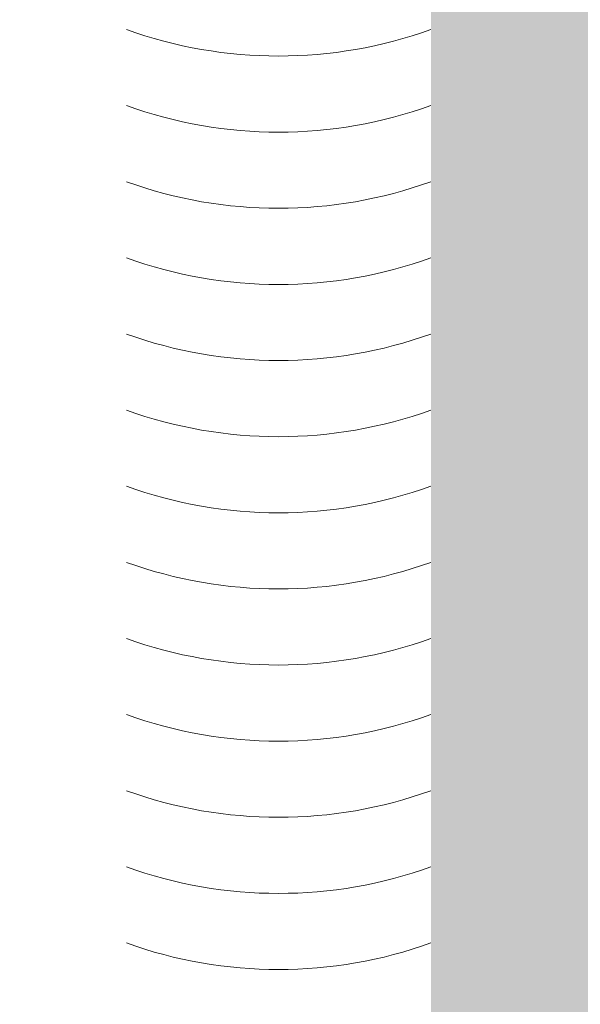
# Model space of a CAD drawing. Units: inches. Extents: x 844 to 2234, y 346 to 1084.
# Tile 17 of 93: x 1114.251 to 1116.421, y 701.25 to 705.06. Entities that reach past the tile are written whole.
import ezdxf

# ---------------------------------------------------------------- set-up
doc = ezdxf.new("R2010")
doc.units = ezdxf.units.IN
doc.header["$MEASUREMENT"] = 0
for name, color, linetype, lineweight in [('A-ANNO-DIMS', 2, 'Continuous', 18), ('furniture', 8, 'Continuous', 18), ('RA-AP-01$0$INT', 35, 'Continuous', 5)]:
    doc.layers.add(name, color=color, linetype=linetype, lineweight=lineweight)
doc.layers.add('RA-AP-01$0$FURN', color=3, linetype='Continuous')
doc.styles.get("Standard").update_dxf_attribs({"font": 'arial.ttf'})
doc.dimstyles.get("Standard").update_dxf_attribs({"dimtxt": 6, "dimasz": 3, "dimexe": 0.18, "dimexo": 0.0625, "dimgap": 0.09, "dimtad": 0, "dimtih": 1, "dimtoh": 1, "dimdec": 1, "dimzin": 0, "dimdsep": 46, "dimlunit": 3, "dimtxsty": 'Standard', "dimblk": 'ARCHTICK', "dimcen": 0.09, "dimadec": 0, "dimazin": 0, "dimtfac": 1, "dimtdec": 1, "dimtofl": 0, "dimtmove": 0, "dimatfit": 3, "dimfxl": 1, "dimtolj": 1, "dimtzin": 0, "dimarcsym": 0})

# ---------------------------------------------------------------- blocks, each defined once
blk = doc.blocks.new('A$C18D01794')
at = {"layer": 'RA-AP-01$0$INT'}
h = blk.add_hatch(color=256, dxfattribs=at)
h.paths.add_polyline_path([(4.355206456958071, -6.156712009588037), (4.355206456958071, -8.056712009588038), (5.455206456958072, -8.056712009588038), (5.455206456958072, -6.156712009588037)])
h.paths.add_polyline_path([(4.405206456958072, -8.006712009588039), (4.405206456958072, -6.206712009588038), (5.405206456958072, -6.206712009588038), (5.405206456958072, -8.006712009588039)], flags=16)
for centre in [(4.309006456954359, -7.648064458284158), (4.309006456951176, -7.671164458284799), (4.309006456954132, -7.671164458285863), (4.309006456953905, -7.694264458283548), (4.309006456953905, -7.717364458282297), (4.309006456952313, -7.740464458286957), (4.30900645695345, -7.763564458285706), (4.30900645695345, -7.786664458281272), (4.309006456951858, -7.80976445828616), (4.309006456950039, -7.832864458284682), (4.309006456952995, -7.855964458280475), (4.309006456952768, -7.879064458285135), (4.309006456951176, -7.902164458283884), (4.309006456949584, -7.925264458285589)]:
    blk.add_arc(centre, 0.136414042854523, 70.20384312815696, 109.7961568705686, dxfattribs=at)
blk = doc.blocks.new('A$C5D2F253E')
at = {"layer": 'RA-AP-01$0$FURN', "xscale": -0.7999999999883585, "yscale": 0.7999999999883585, "zscale": 0.8, "rotation": 90}
blk.add_blockref('A$C18D01794', (-5.687757199772477, 4.75791982714071), dxfattribs=at)
blk = doc.blocks.new('_ArchTick')
at = {"color": 0, "linetype": 'ByBlock', "const_width": 0.15}
blk.add_lwpolyline([(-0.5, -0.5), (0.5, 0.5)], dxfattribs=at)
blk = doc.blocks.new('*D144')
at = {"layer": 'A-ANNO-DIMS', "color": 0, "lineweight": -2, "transparency": 16777216}
for p, q in [((1096.615948, 439.3732739999999), (1096.615948, 1074.743301)), ((1143.115948, 492.373274), (1143.115948, 1074.743301)), ((1096.615948, 1074.563301), (1102.481950728513, 1074.563301)), ((1143.115948, 1074.563301), (1137.249945271487, 1074.563301))]:
    blk.add_line(p, q, dxfattribs=at)
at = {"layer": 'Defpoints', "color": 0, "transparency": 16777216}
for p in [(1143.115948, 1074.563301), (1143.115948, 492.3107739999999), (1096.615948, 439.3107739999999)]:
    blk.add_point(p, dxfattribs=at)
at = {"layer": 'A-ANNO-DIMS', "color": 0, "lineweight": -2, "transparency": 16777216, "xscale": 3, "yscale": 3, "zscale": 3, "rotation": 180}
blk.add_blockref('_ArchTick', (1096.615948, 1074.563301), dxfattribs=at)
at = {"layer": 'A-ANNO-DIMS', "color": 0, "lineweight": -2, "transparency": 16777216, "xscale": 3, "yscale": 3, "zscale": 3}
blk.add_blockref('_ArchTick', (1143.115948, 1074.563301), dxfattribs=at)
at = {"layer": 'A-ANNO-DIMS', "color": 0, "transparency": 16777216, "insert": (1119.865948, 1074.563301), "char_height": 6, "attachment_point": 5}
blk.add_mtext('\\A1;3\'-10 1/2"', dxfattribs=at)

msp = doc.modelspace()

# ---------------------------------------------------------------- block references
at = {"layer": 'furniture', "xscale": 15.94108302203742, "yscale": 15.94108302203742, "zscale": 15.94108302203742, "rotation": 90}
msp.add_blockref('A$C5D2F253E', (1136.147844094663, 696.2584716700112), dxfattribs=at)

# ---------------------------------------------------------------- dimensions: what is measured, and where the dimension line sits
at = {"layer": 'A-ANNO-DIMS'}
dim = msp.add_linear_dim(base=(1143.115948, 1074.563301), p1=(1096.615948, 439.3107739999999), p2=(1143.115948, 492.3107739999999), dimstyle='Standard', override={"dimdec": 1, "dimlfac": 1, "dimrnd": 0, "dimzin": 1, "dimdsep": 46, "dimlunit": 4, "dimfrac": 2}, dxfattribs=at)
dim.commit()
dim.dimension.update_dxf_attribs({"geometry": '*D144', "text_midpoint": (1119.865948, 1074.563301)})

doc.saveas('drawing.dxf')
